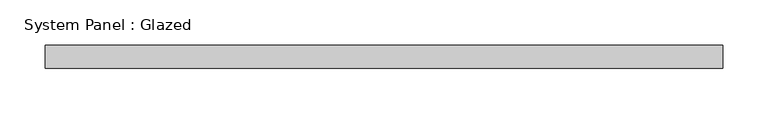
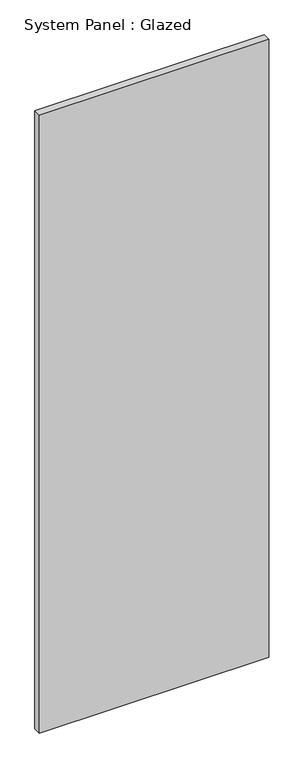
"""IFC4 building model written with IfcOpenShell, lengths in millimetres: plate geometry, System Panel : Glazed."""

from ifc_helpers import new_model, si_unit, origin, origin_with_axes, place, context, project, spatial, polyline, outline, extrude, source, transform, mapped, element, save


def system_panel_glazed_d00a1739(model_context):
    return source(origin(), model_context, "Body", "SweptSolid", [
        extrude(outline(polyline([(374.658438, 19.05), (-374.658438, 19.05), (-374.658438, 44.45), (374.658438, 44.45), (374.658438, 19.05)])), origin_with_axes(), (0.0, 0.0, 1.0), 2132.5340877),
    ])


if __name__ == "__main__":
    model = new_model("IFC4")
    model_context = context("Model", 3, world=origin())
    ifc_project = project(units=[si_unit("LENGTHUNIT", "METRE", prefix="MILLI")], contexts=[model_context])
    site = spatial("IfcSite", under=ifc_project)
    building = spatial("IfcBuilding", under=site)
    placement = place(None, origin())
    system_panel_glazed_shape = system_panel_glazed_d00a1739(model_context)
    element("IfcPlate", 1, ObjectType="System Panel : Glazed", at=placement, inside=building, context=model_context, shape_type="MappedRepresentation", body=[
        mapped(system_panel_glazed_shape, transform((0.0, 0.0, 0.0), x_axis=(1.0, 0.0, 0.0), y_axis=(0.0, 1.0, 0.0), z_axis=(0.0, 0.0, 1.0))),
    ])
    save(model, "model.ifc")

# Revit data of these elements
# Type "System Panel : Glazed"
#   Construction Type Id = "GSP4R"
#   Analytic Construction = "1/8 in Pilkington single glazing"
#   Visual Light Transmittance = 0.9
#   Solar Heat Gain Coefficient = 0.86
#   Heat Transfer Coefficient (U) = 1.18115 BTU/(h·ft²·°F)
# Element 1 (IfcPlate, "System Panel : Glazed")
#   Materials on its faces: "Glass"
# Materials
#   "Glass": class "Glass", colour RGB 0 128 192, transparency 0.75, Description = "Soda Lime Glass", Cost = 0
